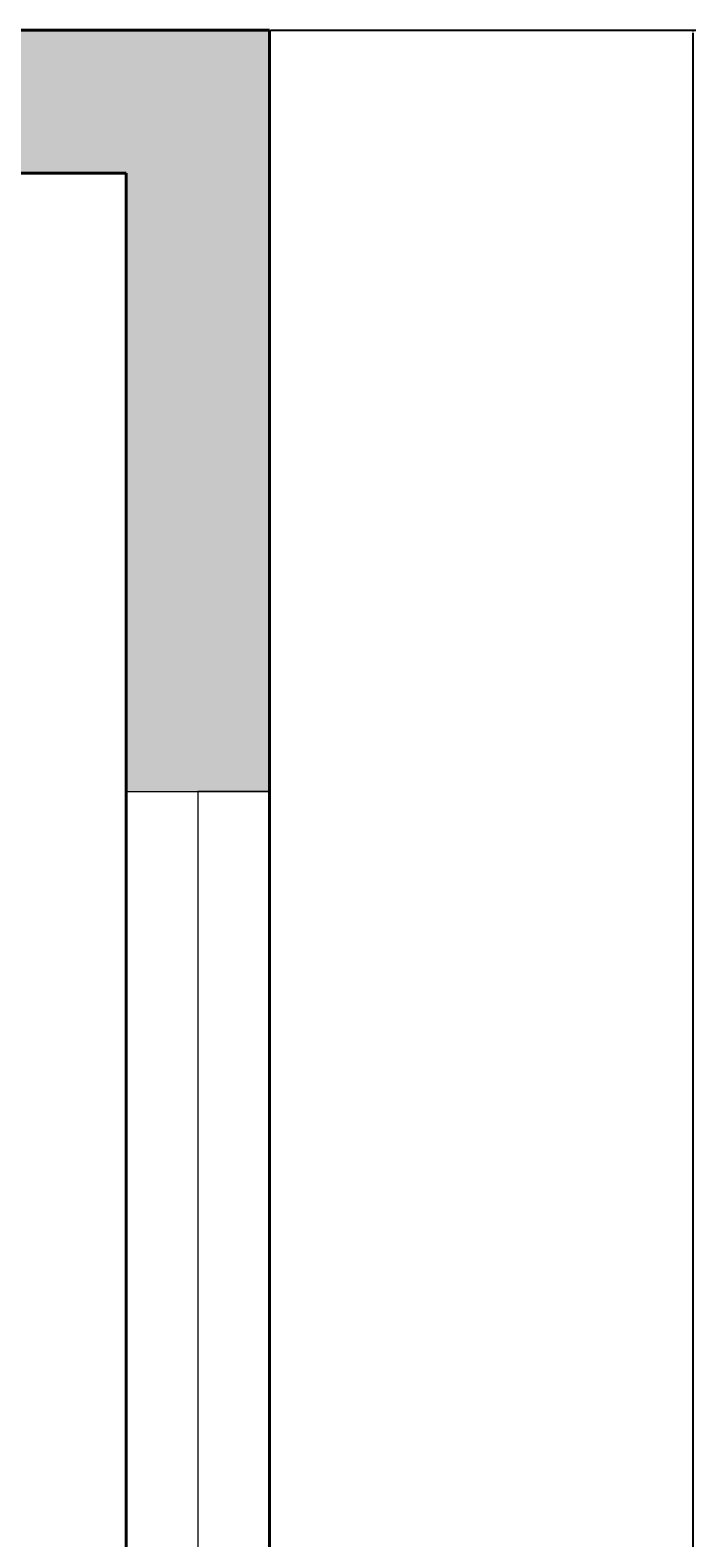
# Model space of a CAD drawing. Units: inches. Extents: x 1441 to 2460, y 1648 to 2683.
# Tile 29 of 35: x 1874 to 1916, y 2204 to 2299. Entities that reach past the tile are written whole.
import ezdxf

# ---------------------------------------------------------------- set-up
doc = ezdxf.new("R2010")
doc.units = ezdxf.units.IN
for name, color, linetype, lineweight in [('A-ANNO-DIMS', 2, 'Continuous', 18), ('A-GLAZ', 4, 'Continuous', 18), ('A-WALL', 7, 'Continuous', 40)]:
    doc.layers.add(name, color=color, linetype=linetype, lineweight=lineweight)
doc.layers.add('A-WALL-PATT', color=251, linetype='Continuous', lineweight=13, true_color=0x636466)
doc.styles.get("Standard").update_dxf_attribs({"font": 'arial.ttf'})
doc.dimstyles.get("Standard").update_dxf_attribs({"dimtxt": 0.18, "dimasz": 0.18, "dimexe": 0.18, "dimexo": 0.0625, "dimgap": 0.09, "dimtad": 0, "dimtih": 1, "dimtoh": 1, "dimdec": 4, "dimzin": 0, "dimdsep": 46, "dimtxsty": 'Standard', "dimcen": 0.09, "dimadec": 0, "dimazin": 0, "dimtfac": 1, "dimtdec": 4, "dimtofl": 0, "dimtmove": 0, "dimatfit": 3, "dimfxl": 1, "dimtolj": 1, "dimtzin": 0, "dimarcsym": 0})

# ---------------------------------------------------------------- blocks, each defined once
blk = doc.blocks.new('WIN-48-SASH')
for p, q in [((8.996, 48.001), (4.496, 48.001)), ((4.496, 48.001), (4.496, 0.001)), ((4.496, 0.001), (-0.004, 0.001))]:
    blk.add_line(p, q)
blk = doc.blocks.new('*D67')
at = {"layer": 'A-ANNO-DIMS', "color": 0, "lineweight": -2, "transparency": 16777216}
for p, q in [((1889.448, 2298.695), (1916.216, 2298.695)), ((1916.036, 2298.515), (1916.036, 2055.938)), ((1916.036, 1812.997), (1916.036, 2055.574)), ((1758.224, 1812.817), (1916.216, 1812.817))]:
    blk.add_line(p, q, dxfattribs=at)
at = {"layer": 'A-ANNO-DIMS', "color": 0, "transparency": 16777216}
for points in [[(1916.006, 2298.515), (1916.066, 2298.515), (1916.036, 2298.695)], [(1916.006, 1812.997), (1916.066, 1812.997), (1916.036, 1812.817)]]:
    blk.add_solid(points, dxfattribs=at)
at = {"layer": 'Defpoints', "color": 0, "transparency": 16777216}
for p in [(1889.386, 2298.695), (1916.036, 2298.695), (1758.161, 1812.817)]:
    blk.add_point(p, dxfattribs=at)
at = {"layer": 'A-ANNO-DIMS', "color": 0, "transparency": 16777216, "insert": (1916.036, 2055.756), "char_height": 0.18, "attachment_point": 5}
blk.add_mtext('\\A1;485.9', dxfattribs=at)

msp = doc.modelspace()

# ---------------------------------------------------------------- hatches: boundary and pattern name
at = {"layer": 'A-WALL-PATT'}
h = msp.add_hatch(color=256, dxfattribs=at)
h.dxf.hatch_style = 1
h.paths.add_polyline_path([(1627.5085, 2298.6952), (1568.8859, 2298.6952), (1568.8859, 2246.9605), (1577.8859, 2246.9605), (1577.8859, 2289.6952), (1627.5085, 2289.6952), (1627.5085, 2294.1952)])
h.paths.add_polyline_path([(1675.5777, 2298.6952), (1651.5085, 2298.6952), (1651.5085, 2289.6952), (1675.5777, 2289.6952), (1675.5777, 2294.1952)])
h.paths.add_polyline_path([(1667.3859, 2289.6952), (1662.8859, 2289.6952), (1662.8859, 2233.0622), (1667.3859, 2233.0622)])
h.paths.add_polyline_path([(1715.8721, 2294.3362), (1715.8721, 2295.2788), (1715.8721, 2298.6952), (1699.5777, 2298.6952), (1699.5777, 2289.6952), (1715.8721, 2289.6952)])
h.paths.add_polyline_path([(1707.8859, 2289.6952), (1703.3859, 2289.6952), (1703.3859, 2199.6952), (1707.8859, 2199.6952)])
h.paths.add_polyline_path([(1760.3859, 2204.637), (1755.8859, 2204.637), (1755.8859, 2199.6952), (1667.3859, 2199.6952), (1667.3859, 2204.637), (1662.8859, 2204.637), (1662.8859, 2195.1952), (1760.3859, 2195.1952)])
h.paths.add_polyline_path([(1760.3859, 2289.6952), (1755.8859, 2289.6952), (1755.8859, 2233.0622), (1760.3859, 2233.0622)])
h.paths.add_polyline_path([(1889.3859, 2298.6952), (1739.8721, 2298.6952), (1739.8721, 2289.6952), (1880.3859, 2289.6952), (1880.3859, 2250.8051), (1889.3859, 2250.8051)])
h.paths.add_polyline_path([(1889.3859, 2202.8051), (1880.3859, 2202.8051), (1880.3859, 2157.6952), (1747.948, 2157.6952), (1747.948, 2153.1952), (1755.8859, 2153.1952), (1755.8859, 2058.005), (1760.3859, 2058.005), (1760.3859, 2153.1952), (1880.3859, 2153.1952), (1880.3859, 2124.108), (1889.3859, 2124.108)])
h.paths.add_polyline_path([(1889.3859, 1984.8305), (1880.3859, 1984.8305), (1880.3859, 1834.1952), (1889.3859, 1834.1952)])
h.paths.add_polyline_path([(1889.3859, 2076.108), (1880.3859, 2076.108), (1880.3859, 2008.8305), (1889.3859, 2008.8305)])
h.paths.add_polyline_path([(1880.3859, 2027.1952), (1800.8859, 2027.1952), (1800.8859, 2000.9452), (1805.3859, 2000.9452), (1805.3859, 2022.6952), (1880.3859, 2022.6952)])
h.paths.add_polyline_path([(1800.8859, 2027.1952), (1760.3859, 2027.1952), (1760.3859, 2030.7912), (1755.8859, 2030.7912), (1755.8859, 2022.6952), (1800.8859, 2022.6952)])
h.paths.add_polyline_path([(1880.3859, 1974.6952), (1805.3859, 1974.6952), (1805.3859, 1978.7973), (1800.8859, 1978.7973), (1800.8859, 1974.6952), (1794.8823, 1974.6952), (1794.8823, 1970.1952), (1800.8859, 1970.1952), (1805.3859, 1970.1952), (1880.3859, 1970.1952)])
h.paths.add_polyline_path([(1760.3859, 1974.6952), (1755.8859, 1974.6952), (1755.8859, 1925.6952), (1751.8616, 1925.6952), (1751.8616, 1921.1952), (1760.3859, 1921.1952)])
h.paths.add_polyline_path([(1760.3859, 1921.1952), (1755.8859, 1921.1952), (1755.8859, 1843.1952), (1760.3859, 1843.1952)])
h.paths.add_polyline_path([(1799.1136, 1838.6952), (1799.1136, 1843.1952), (1760.3859, 1843.1952), (1751.8944, 1843.1952), (1751.8944, 1834.1952), (1758.1615, 1834.1952), (1799.1136, 1834.1952)])
h.paths.add_polyline_path([(1880.3859, 1843.1952), (1859.1136, 1843.1952), (1859.1136, 1834.1952), (1880.3859, 1834.1952)])
h.paths.add_polyline_path([(1577.8859, 1857.7914), (1568.8859, 1857.7914), (1568.8859, 1834.1952), (1695.0034, 1834.1952), (1695.0034, 1838.6952), (1695.0034, 1843.1952), (1577.8859, 1843.1952)])
h.paths.add_polyline_path([(1577.8859, 1959.2399), (1573.3859, 1959.2399), (1568.8859, 1959.2399), (1568.8859, 1905.7914), (1577.8859, 1905.7914), (1577.8859, 1921.1952), (1703.3859, 1921.1952), (1707.8859, 1921.1952), (1715.1501, 1921.1952), (1715.1501, 1925.6952), (1707.8859, 1925.6952), (1703.3859, 1925.6952), (1577.8859, 1925.6952)])
h.paths.add_polyline_path([(1577.8859, 2106.6907), (1568.8859, 2106.6907), (1568.8859, 2019.2399), (1577.8859, 2019.2399)])
h.paths.add_polyline_path([(1707.8859, 2051.6952), (1703.3859, 2051.6952), (1703.3859, 2048.6952), (1703.3859, 1925.6952), (1707.8859, 1925.6952)])
h.paths.add_polyline_path([(1703.3859, 2051.6952), (1676.3859, 2051.6952), (1676.3859, 2048.6952), (1703.3859, 2048.6952)])
h.paths.add_polyline_path([(1703.3859, 2102.6952), (1676.3859, 2102.6952), (1676.3859, 2099.6952), (1685.3859, 2099.6952), (1703.3859, 2099.6952)])
h.paths.add_polyline_path([(1707.8859, 2153.1952), (1710.5611, 2153.1952), (1710.5611, 2157.6952), (1707.8859, 2157.6952), (1707.8859, 2195.1952), (1703.3859, 2195.1952), (1703.3859, 2099.6952), (1707.8859, 2099.6952)])
h.paths.add_polyline_path([(1577.8859, 2198.9605), (1568.8859, 2198.9605), (1568.8859, 2166.6907), (1577.8859, 2166.6907)])

# ---------------------------------------------------------------- linework, layer by layer
at = {"layer": 'A-GLAZ'}
msp.add_line((1880.3859, 2250.8051), (1889.3859, 2250.8051), dxfattribs=at)
at = {"layer": 'A-WALL'}
for p, q in [((1568.8859, 2298.6952), (1889.3859, 2298.6952)), ((1889.3859, 2298.6952), (1889.3859, 1834.1952)), ((1577.8859, 2289.6952), (1880.3859, 2289.6952)), ((1880.3859, 2289.6952), (1880.3859, 2157.6952))]:
    msp.add_line(p, q, dxfattribs=at)

# ---------------------------------------------------------------- block references
at = {"layer": 'A-GLAZ'}
msp.add_blockref('WIN-48-SASH', (1880.39, 2202.8045), dxfattribs=at)

# ---------------------------------------------------------------- dimensions: what is measured, and where the dimension line sits
at = {"layer": 'A-ANNO-DIMS'}
dim = msp.add_linear_dim(base=(1916.0359, 2298.6952), p1=(1758.1615, 1812.8171), p2=(1889.3859, 2298.6952), angle=90, dimstyle='Standard', override={"dimdec": 1, "dimlfac": 1, "dimrnd": 0, "dimzin": 0, "dimdsep": 46, "dimlunit": 2}, dxfattribs=at)
dim.commit()
dim.dimension.update_dxf_attribs({"geometry": '*D67', "text_midpoint": (1916.0359, 2055.7561)})

doc.saveas('drawing.dxf')
